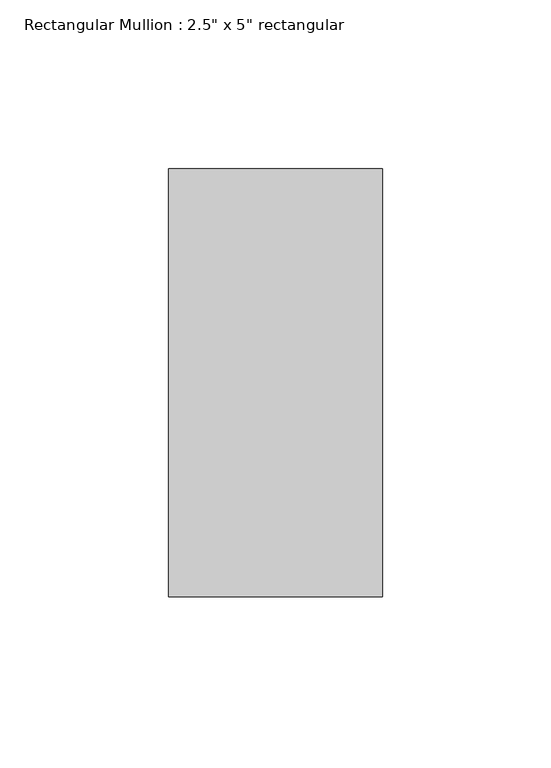
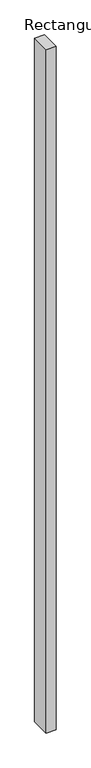
"""IFC4 building model written with IfcOpenShell, lengths in millimetres: member geometry."""

from ifc_helpers import new_model, si_unit, frame, origin, place, context, project, spatial, polyline, outline, extrude, source, transform, mapped, element, save


def member_5c8c9790(model_context):
    return source(origin(), model_context, "Body", "SweptSolid", [
        extrude(outline(polyline([(0.0, 63.5), (0.0, -63.5), (-63.5, -63.5), (-63.5, 63.5), (0.0, 63.5)])), frame((0.0, 0.0, -4629.15), z_axis=(0.0, 0.0, 1.0), x_axis=(1.0, 0.0, 0.0)), (0.0, 0.0, 1.0), 4629.15),
    ])


if __name__ == "__main__":
    model = new_model("IFC4")
    model_context = context("Model", 3, world=origin())
    ifc_project = project(units=[si_unit("LENGTHUNIT", "METRE", prefix="MILLI")], contexts=[model_context])
    site = spatial("IfcSite", under=ifc_project)
    building = spatial("IfcBuilding", under=site)
    placement = place(None, origin())
    member_shape = member_5c8c9790(model_context)
    element("IfcMember", 1, ObjectType="Rectangular Mullion : 2.5\" x 5\" rectangular", at=placement, inside=building, context=model_context, shape_type="MappedRepresentation", body=[
        mapped(member_shape, transform((0.0, 0.0, 0.0), x_axis=(1.0, 0.0, 0.0), y_axis=(0.0, 1.0, 0.0), z_axis=(0.0, 0.0, 1.0))),
    ])
    save(model, "model.ifc")

# Revit data of these elements
# Type "Rectangular Mullion : 2.5\" x 5\" rectangular"
#   built-in parameter 1007304 = 0.416667 (stored number, unit not read)
#   built-in parameter 1007301 = 0.104167 (stored number, unit not read)
#   built-in parameter 1007300 = 0.104167 (stored number, unit not read)
# Element 1 (IfcMember, "Rectangular Mullion : 2.5\" x 5\" rectangular")
#   Materials on its faces: "Aluminum"
# Materials
#   "Aluminum": class "Metal", colour RGB 247 247 247, transparency 0, Description = "Aluminum 6061", Cost = 0
